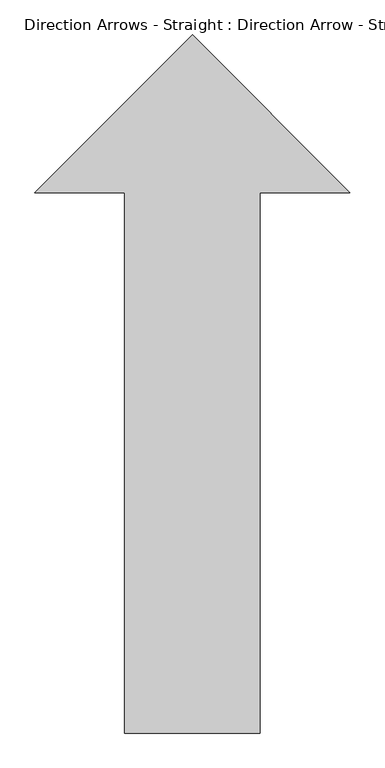
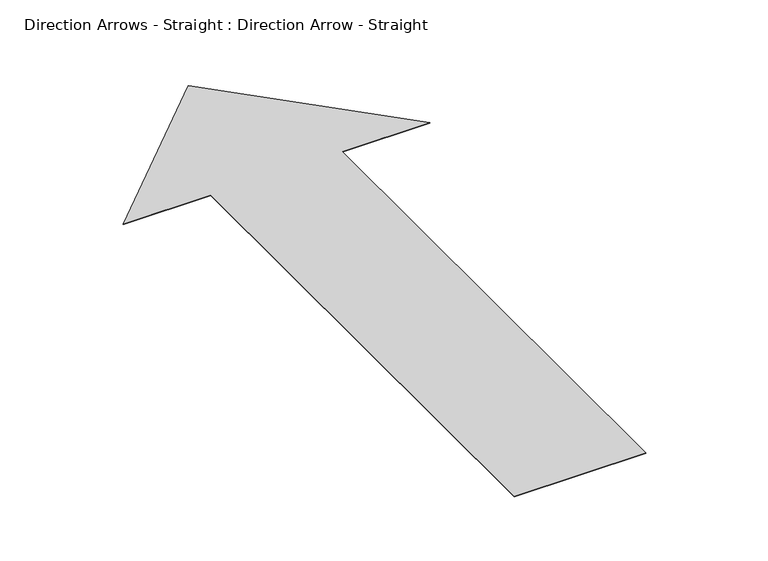
"""IFC4 building model written with IfcOpenShell, lengths in millimetres: geographic element geometry, Direction Arrows - Straight : Direction Arrow - Straight."""

from ifc_helpers import new_model, si_unit, origin, origin_with_axes, place, context, project, spatial, polyline, outline, extrude, source, transform, mapped, element, save


def direction_arrows_straight_direction_arrow_straight_a0d3235c(model_context):
    return source(origin(), model_context, "Body", "SweptSolid", [
        extrude(outline(polyline([(0.0, 1574.8), (355.6, 1219.2), (152.4, 1219.2), (152.4, 0.0), (-152.4, 0.0), (-152.4, 1219.2), (-355.6, 1219.2), (0.0, 1574.8)])), origin_with_axes(), (0.0, 0.0, 1.0), 1.5875),
    ])


if __name__ == "__main__":
    model = new_model("IFC4")
    model_context = context("Model", 3, world=origin())
    ifc_project = project(units=[si_unit("LENGTHUNIT", "METRE", prefix="MILLI")], contexts=[model_context])
    site = spatial("IfcSite", under=ifc_project)
    building = spatial("IfcBuilding", under=site)
    placement = place(None, origin())
    direction_arrows_straight_direction_arrow_straight_shape = direction_arrows_straight_direction_arrow_straight_a0d3235c(model_context)
    element("IfcGeographicElement", 1, ObjectType="Direction Arrows - Straight : Direction Arrow - Straight", at=placement, inside=building, context=model_context, shape_type="MappedRepresentation", body=[
        mapped(direction_arrows_straight_direction_arrow_straight_shape, transform((0.0, 0.0, 0.0), x_axis=(1.0, 0.0, 0.0), y_axis=(0.0, 1.0, 0.0), z_axis=(0.0, 0.0, 1.0))),
    ])
    save(model, "model.ifc")

# Revit data of these elements
# Element 1 (IfcGeographicElement, "Direction Arrows - Straight : Direction Arrow - Straight")
#   Materials on its faces: "Paint - White"
# Materials
#   "Paint - White": class "Paint", colour RGB 249 249 249, transparency 0
